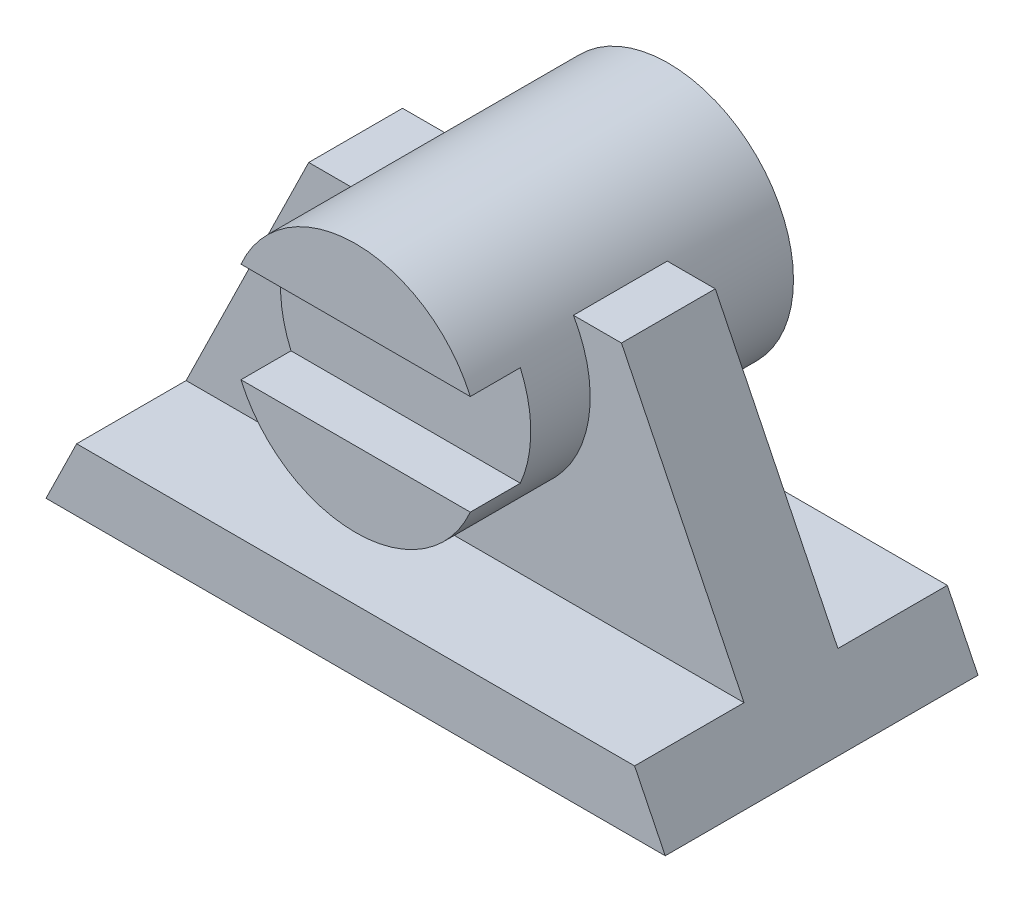
ISO-10303-21;
HEADER;
FILE_DESCRIPTION(('STEP AP214'),'2;1');
FILE_NAME('part.step','',(''),(''),'','','');
FILE_SCHEMA(('AUTOMOTIVE_DESIGN { 1 0 10303 214 1 1 1 1 }'));
ENDSEC;
DATA;
#1=APPLICATION_CONTEXT('core data for automotive mechanical design processes');
#2=APPLICATION_PROTOCOL_DEFINITION('international standard','automotive_design',2000,#1);
#3=PRODUCT_CONTEXT('',#1,'mechanical');
#4=PRODUCT('Part','Part','',(#3));
#5=PRODUCT_RELATED_PRODUCT_CATEGORY('part','',(#4));
#6=PRODUCT_DEFINITION_FORMATION('','',#4);
#7=PRODUCT_DEFINITION_CONTEXT('part definition',#1,'design');
#8=PRODUCT_DEFINITION('design','',#6,#7);
#9=PRODUCT_DEFINITION_SHAPE('','',#8);
#10=(LENGTH_UNIT() NAMED_UNIT(*) SI_UNIT(.MILLI.,.METRE.));
#11=(NAMED_UNIT(*) PLANE_ANGLE_UNIT() SI_UNIT($,.RADIAN.));
#12=(NAMED_UNIT(*) SI_UNIT($,.STERADIAN.) SOLID_ANGLE_UNIT());
#13=UNCERTAINTY_MEASURE_WITH_UNIT(LENGTH_MEASURE(1.E-05),#10,'distance_accuracy_value','');
#14=(GEOMETRIC_REPRESENTATION_CONTEXT(3) GLOBAL_UNCERTAINTY_ASSIGNED_CONTEXT((#13)) GLOBAL_UNIT_ASSIGNED_CONTEXT((#10,
#11,#12)) REPRESENTATION_CONTEXT('',''));
#15=CARTESIAN_POINT('',(0.,0.,0.));
#16=DIRECTION('',(0.,0.,1.));
#17=DIRECTION('',(1.,0.,0.));
#18=AXIS2_PLACEMENT_3D('',#15,#16,#17);
#19=CARTESIAN_POINT('',(0.,40.,25.));
#20=DIRECTION('',(0.,0.,1.));
#21=DIRECTION('',(1.,0.,0.));
#22=AXIS2_PLACEMENT_3D('',#19,#20,#21);
#23=PLANE('',#22);
#24=DIRECTION('',(-1.,0.,0.));
#25=VECTOR('',#24,1.);
#26=CARTESIAN_POINT('',(-23.6638655462185,48.,25.));
#27=LINE('',#26,#25);
#28=CARTESIAN_POINT('',(18.3303027798234,48.,25.));
#29=VERTEX_POINT('',#28);
#30=CARTESIAN_POINT('',(-18.3303027798234,48.,25.));
#31=VERTEX_POINT('',#30);
#32=EDGE_CURVE('E141',#29,#31,#27,.T.);
#33=ORIENTED_EDGE('',*,*,#32,.F.);
#34=CARTESIAN_POINT('',(0.,40.,25.));
#35=DIRECTION('',(0.,0.,1.));
#36=DIRECTION('',(1.,0.,0.));
#37=AXIS2_PLACEMENT_3D('',#34,#35,#36);
#38=CIRCLE('',#37,20.);
#39=EDGE_CURVE('E153',#29,#31,#38,.T.);
#40=ORIENTED_EDGE('',*,*,#39,.T.);
#41=EDGE_LOOP('',(#33,#40));
#42=FACE_BOUND('',#41,.T.);
#43=ADVANCED_FACE('F39',(#42),#23,.T.);
#44=CARTESIAN_POINT('',(0.,50.,0.));
#45=DIRECTION('',(0.,1.,0.));
#46=DIRECTION('',(0.,0.,1.));
#47=AXIS2_PLACEMENT_3D('',#44,#45,#46);
#48=PLANE('',#47);
#49=DIRECTION('',(-1.,0.,0.));
#50=VECTOR('',#49,1.);
#51=CARTESIAN_POINT('',(-49.5,50.,-7.50000000000001));
#52=LINE('',#51,#50);
#53=CARTESIAN_POINT('',(25.,50.,-7.50000000000001));
#54=VERTEX_POINT('',#53);
#55=CARTESIAN_POINT('',(17.3205080756888,50.,-7.50000000000001));
#56=VERTEX_POINT('',#55);
#57=EDGE_CURVE('E220',#54,#56,#52,.T.);
#58=ORIENTED_EDGE('',*,*,#57,.T.);
#59=DIRECTION('',(0.,0.,-1.));
#60=VECTOR('',#59,1.);
#61=CARTESIAN_POINT('',(17.3205080756888,50.,25.));
#62=LINE('',#61,#60);
#63=CARTESIAN_POINT('',(17.3205080756888,50.,7.49999999999999));
#64=VERTEX_POINT('',#63);
#65=EDGE_CURVE('E62',#56,#64,#62,.F.);
#66=ORIENTED_EDGE('',*,*,#65,.T.);
#67=DIRECTION('',(1.,0.,0.));
#68=VECTOR('',#67,1.);
#69=CARTESIAN_POINT('',(-49.5,50.,7.49999999999999));
#70=LINE('',#69,#68);
#71=CARTESIAN_POINT('',(25.,50.,7.49999999999999));
#72=VERTEX_POINT('',#71);
#73=EDGE_CURVE('E217',#64,#72,#70,.T.);
#74=ORIENTED_EDGE('',*,*,#73,.T.);
#75=DIRECTION('',(0.,0.,1.));
#76=VECTOR('',#75,1.);
#77=CARTESIAN_POINT('',(25.,50.,-40.));
#78=LINE('',#77,#76);
#79=EDGE_CURVE('E177',#54,#72,#78,.T.);
#80=ORIENTED_EDGE('',*,*,#79,.F.);
#81=EDGE_LOOP('',(#58,#66,#74,#80));
#82=FACE_BOUND('',#81,.T.);
#83=ADVANCED_FACE('F274',(#82),#48,.T.);
#84=CARTESIAN_POINT('',(-25.,50.,7.49999999999999));
#85=VERTEX_POINT('',#84);
#86=CARTESIAN_POINT('',(-17.3205080756888,50.,7.49999999999999));
#87=VERTEX_POINT('',#86);
#88=EDGE_CURVE('E215',#85,#87,#70,.T.);
#89=ORIENTED_EDGE('',*,*,#88,.T.);
#90=DIRECTION('',(0.,0.,-1.));
#91=VECTOR('',#90,1.);
#92=CARTESIAN_POINT('',(-17.3205080756888,50.,25.));
#93=LINE('',#92,#91);
#94=CARTESIAN_POINT('',(-17.3205080756888,50.,-7.50000000000001));
#95=VERTEX_POINT('',#94);
#96=EDGE_CURVE('E162',#87,#95,#93,.T.);
#97=ORIENTED_EDGE('',*,*,#96,.T.);
#98=CARTESIAN_POINT('',(-25.,50.,-7.50000000000001));
#99=VERTEX_POINT('',#98);
#100=EDGE_CURVE('E213',#95,#99,#52,.T.);
#101=ORIENTED_EDGE('',*,*,#100,.T.);
#102=DIRECTION('',(0.,0.,1.));
#103=VECTOR('',#102,1.);
#104=CARTESIAN_POINT('',(-25.,50.,-40.));
#105=LINE('',#104,#103);
#106=EDGE_CURVE('E179',#99,#85,#105,.T.);
#107=ORIENTED_EDGE('',*,*,#106,.T.);
#108=EDGE_LOOP('',(#89,#97,#101,#107));
#109=FACE_BOUND('',#108,.T.);
#110=ADVANCED_FACE('F279',(#109),#48,.T.);
#111=CARTESIAN_POINT('',(0.,10.,0.));
#112=DIRECTION('',(0.,1.,0.));
#113=DIRECTION('',(0.,0.,1.));
#114=AXIS2_PLACEMENT_3D('',#111,#112,#113);
#115=PLANE('',#114);
#116=DIRECTION('',(0.,0.,-1.));
#117=VECTOR('',#116,1.);
#118=CARTESIAN_POINT('',(-44.6,10.,0.));
#119=LINE('',#118,#117);
#120=CARTESIAN_POINT('',(-44.6,10.,-7.50000000000001));
#121=VERTEX_POINT('',#120);
#122=CARTESIAN_POINT('',(-44.6,10.,-25.));
#123=VERTEX_POINT('',#122);
#124=EDGE_CURVE('E199',#121,#123,#119,.T.);
#125=ORIENTED_EDGE('',*,*,#124,.F.);
#126=DIRECTION('',(-1.,0.,0.));
#127=VECTOR('',#126,1.);
#128=CARTESIAN_POINT('',(-49.5,10.,-7.50000000000001));
#129=LINE('',#128,#127);
#130=CARTESIAN_POINT('',(44.6,9.99999999999999,-7.50000000000001));
#131=VERTEX_POINT('',#130);
#132=EDGE_CURVE('E225',#131,#121,#129,.T.);
#133=ORIENTED_EDGE('',*,*,#132,.F.);
#134=DIRECTION('',(0.,0.,1.));
#135=VECTOR('',#134,1.);
#136=CARTESIAN_POINT('',(44.6,10.,0.));
#137=LINE('',#136,#135);
#138=CARTESIAN_POINT('',(44.6,10.,-25.));
#139=VERTEX_POINT('',#138);
#140=EDGE_CURVE('E182',#139,#131,#137,.T.);
#141=ORIENTED_EDGE('',*,*,#140,.F.);
#142=DIRECTION('',(-1.,0.,0.));
#143=VECTOR('',#142,1.);
#144=CARTESIAN_POINT('',(-49.5,10.,-25.));
#145=LINE('',#144,#143);
#146=EDGE_CURVE('E223',#139,#123,#145,.T.);
#147=ORIENTED_EDGE('',*,*,#146,.T.);
#148=EDGE_LOOP('',(#125,#133,#141,#147));
#149=FACE_BOUND('',#148,.T.);
#150=ADVANCED_FACE('F281',(#149),#115,.T.);
#151=CARTESIAN_POINT('',(-49.5,10.,-25.));
#152=DIRECTION('',(0.,0.,1.));
#153=DIRECTION('',(1.,0.,0.));
#154=AXIS2_PLACEMENT_3D('',#151,#152,#153);
#155=PLANE('',#154);
#156=DIRECTION('',(-1.,0.,0.));
#157=VECTOR('',#156,1.);
#158=CARTESIAN_POINT('',(-49.5,0.,-25.));
#159=LINE('',#158,#157);
#160=CARTESIAN_POINT('',(49.5,0.,-25.));
#161=VERTEX_POINT('',#160);
#162=CARTESIAN_POINT('',(-49.5,0.,-25.));
#163=VERTEX_POINT('',#162);
#164=EDGE_CURVE('E234',#161,#163,#159,.T.);
#165=ORIENTED_EDGE('',*,*,#164,.T.);
#166=DIRECTION('',(0.440015247772983,0.897990301577517,0.));
#167=VECTOR('',#166,1.);
#168=CARTESIAN_POINT('',(-45.5487057495363,8.0638658172728,-25.));
#169=LINE('',#168,#167);
#170=EDGE_CURVE('E198',#163,#123,#169,.T.);
#171=ORIENTED_EDGE('',*,*,#170,.T.);
#172=ORIENTED_EDGE('',*,*,#146,.F.);
#173=DIRECTION('',(0.440015247772983,-0.897990301577517,0.));
#174=VECTOR('',#173,1.);
#175=CARTESIAN_POINT('',(26.3809773405371,47.1816788968632,-25.));
#176=LINE('',#175,#174);
#177=EDGE_CURVE('E190',#139,#161,#176,.T.);
#178=ORIENTED_EDGE('',*,*,#177,.T.);
#179=EDGE_LOOP('',(#165,#171,#172,#178));
#180=FACE_BOUND('',#179,.T.);
#181=ADVANCED_FACE('F41',(#180),#155,.F.);
#182=CARTESIAN_POINT('',(-49.5,10.,25.));
#183=DIRECTION('',(0.,0.,-1.));
#184=DIRECTION('',(-1.,0.,0.));
#185=AXIS2_PLACEMENT_3D('',#182,#183,#184);
#186=PLANE('',#185);
#187=DIRECTION('',(1.,0.,0.));
#188=VECTOR('',#187,1.);
#189=CARTESIAN_POINT('',(-49.5,10.,25.));
#190=LINE('',#189,#188);
#191=CARTESIAN_POINT('',(-44.6,10.,25.));
#192=VERTEX_POINT('',#191);
#193=CARTESIAN_POINT('',(44.6,10.,25.));
#194=VERTEX_POINT('',#193);
#195=EDGE_CURVE('E226',#192,#194,#190,.T.);
#196=ORIENTED_EDGE('',*,*,#195,.F.);
#197=DIRECTION('',(-0.440015247772983,-0.897990301577517,0.));
#198=VECTOR('',#197,1.);
#199=CARTESIAN_POINT('',(-45.5487057495363,8.06386581727281,25.));
#200=LINE('',#199,#198);
#201=CARTESIAN_POINT('',(-49.5,0.,25.));
#202=VERTEX_POINT('',#201);
#203=EDGE_CURVE('E206',#192,#202,#200,.T.);
#204=ORIENTED_EDGE('',*,*,#203,.T.);
#205=DIRECTION('',(1.,0.,0.));
#206=VECTOR('',#205,1.);
#207=CARTESIAN_POINT('',(-49.5,0.,25.));
#208=LINE('',#207,#206);
#209=CARTESIAN_POINT('',(49.5,0.,25.));
#210=VERTEX_POINT('',#209);
#211=EDGE_CURVE('E230',#202,#210,#208,.T.);
#212=ORIENTED_EDGE('',*,*,#211,.T.);
#213=DIRECTION('',(-0.440015247772983,0.897990301577517,0.));
#214=VECTOR('',#213,1.);
#215=CARTESIAN_POINT('',(26.3809773405371,47.1816788968631,25.));
#216=LINE('',#215,#214);
#217=EDGE_CURVE('E193',#210,#194,#216,.T.);
#218=ORIENTED_EDGE('',*,*,#217,.T.);
#219=EDGE_LOOP('',(#196,#204,#212,#218));
#220=FACE_BOUND('',#219,.T.);
#221=ADVANCED_FACE('F305',(#220),#186,.F.);
#222=DIRECTION('',(0.,0.,-1.));
#223=VECTOR('',#222,1.);
#224=CARTESIAN_POINT('',(-44.6,10.,0.));
#225=LINE('',#224,#223);
#226=CARTESIAN_POINT('',(-44.6,10.,7.49999999999999));
#227=VERTEX_POINT('',#226);
#228=EDGE_CURVE('E207',#192,#227,#225,.T.);
#229=ORIENTED_EDGE('',*,*,#228,.F.);
#230=ORIENTED_EDGE('',*,*,#195,.T.);
#231=DIRECTION('',(0.,0.,1.));
#232=VECTOR('',#231,1.);
#233=CARTESIAN_POINT('',(44.6,10.,0.));
#234=LINE('',#233,#232);
#235=CARTESIAN_POINT('',(44.6,9.99999999999999,7.49999999999999));
#236=VERTEX_POINT('',#235);
#237=EDGE_CURVE('E194',#236,#194,#234,.T.);
#238=ORIENTED_EDGE('',*,*,#237,.F.);
#239=DIRECTION('',(1.,0.,0.));
#240=VECTOR('',#239,1.);
#241=CARTESIAN_POINT('',(-49.5,10.,7.49999999999999));
#242=LINE('',#241,#240);
#243=EDGE_CURVE('E212',#227,#236,#242,.T.);
#244=ORIENTED_EDGE('',*,*,#243,.F.);
#245=EDGE_LOOP('',(#229,#230,#238,#244));
#246=FACE_BOUND('',#245,.T.);
#247=ADVANCED_FACE('F299',(#246),#115,.T.);
#248=CARTESIAN_POINT('',(0.,0.,0.));
#249=DIRECTION('',(0.,1.,0.));
#250=DIRECTION('',(0.,0.,1.));
#251=AXIS2_PLACEMENT_3D('',#248,#249,#250);
#252=PLANE('',#251);
#253=DIRECTION('',(0.,0.,-1.));
#254=VECTOR('',#253,1.);
#255=CARTESIAN_POINT('',(49.5,0.,-25.));
#256=LINE('',#255,#254);
#257=EDGE_CURVE('E216',#210,#161,#256,.T.);
#258=ORIENTED_EDGE('',*,*,#257,.F.);
#259=ORIENTED_EDGE('',*,*,#211,.F.);
#260=DIRECTION('',(0.,0.,1.));
#261=VECTOR('',#260,1.);
#262=CARTESIAN_POINT('',(-49.5,0.,-25.));
#263=LINE('',#262,#261);
#264=EDGE_CURVE('E240',#163,#202,#263,.T.);
#265=ORIENTED_EDGE('',*,*,#264,.F.);
#266=ORIENTED_EDGE('',*,*,#164,.F.);
#267=EDGE_LOOP('',(#258,#259,#265,#266));
#268=FACE_BOUND('',#267,.T.);
#269=ADVANCED_FACE('F300',(#268),#252,.F.);
#270=CARTESIAN_POINT('',(-49.5,50.,7.49999999999999));
#271=DIRECTION('',(0.,0.,-1.));
#272=DIRECTION('',(-1.,0.,0.));
#273=AXIS2_PLACEMENT_3D('',#270,#271,#272);
#274=PLANE('',#273);
#275=CARTESIAN_POINT('',(0.,40.,7.49999999999999));
#276=DIRECTION('',(0.,0.,-1.));
#277=DIRECTION('',(-1.,0.,0.));
#278=AXIS2_PLACEMENT_3D('',#275,#276,#277);
#279=CIRCLE('',#278,20.);
#280=EDGE_CURVE('E176',#87,#64,#279,.F.);
#281=ORIENTED_EDGE('',*,*,#280,.F.);
#282=ORIENTED_EDGE('',*,*,#88,.F.);
#283=DIRECTION('',(-0.440015247772983,-0.897990301577517,0.));
#284=VECTOR('',#283,1.);
#285=CARTESIAN_POINT('',(-29.7435287476816,40.319329086364,7.49999999999999));
#286=LINE('',#285,#284);
#287=EDGE_CURVE('E204',#85,#227,#286,.T.);
#288=ORIENTED_EDGE('',*,*,#287,.T.);
#289=ORIENTED_EDGE('',*,*,#243,.T.);
#290=DIRECTION('',(-0.440015247772983,0.897990301577517,0.));
#291=VECTOR('',#290,1.);
#292=CARTESIAN_POINT('',(10.5758003386824,79.4371421659544,7.49999999999999));
#293=LINE('',#292,#291);
#294=EDGE_CURVE('E188',#236,#72,#293,.T.);
#295=ORIENTED_EDGE('',*,*,#294,.T.);
#296=ORIENTED_EDGE('',*,*,#73,.F.);
#297=EDGE_LOOP('',(#281,#282,#288,#289,#295,#296));
#298=FACE_BOUND('',#297,.T.);
#299=ADVANCED_FACE('F291',(#298),#274,.F.);
#300=CARTESIAN_POINT('',(-49.5,50.,-7.50000000000001));
#301=DIRECTION('',(0.,0.,1.));
#302=DIRECTION('',(1.,0.,0.));
#303=AXIS2_PLACEMENT_3D('',#300,#301,#302);
#304=PLANE('',#303);
#305=CARTESIAN_POINT('',(0.,40.,-7.50000000000001));
#306=DIRECTION('',(0.,0.,1.));
#307=DIRECTION('',(1.,0.,0.));
#308=AXIS2_PLACEMENT_3D('',#305,#306,#307);
#309=CIRCLE('',#308,20.);
#310=EDGE_CURVE('E244',#56,#95,#309,.F.);
#311=ORIENTED_EDGE('',*,*,#310,.F.);
#312=ORIENTED_EDGE('',*,*,#57,.F.);
#313=DIRECTION('',(0.440015247772983,-0.897990301577517,0.));
#314=VECTOR('',#313,1.);
#315=CARTESIAN_POINT('',(10.5758003386824,79.4371421659544,-7.50000000000001));
#316=LINE('',#315,#314);
#317=EDGE_CURVE('E235',#54,#131,#316,.T.);
#318=ORIENTED_EDGE('',*,*,#317,.T.);
#319=ORIENTED_EDGE('',*,*,#132,.T.);
#320=DIRECTION('',(0.440015247772983,0.897990301577517,0.));
#321=VECTOR('',#320,1.);
#322=CARTESIAN_POINT('',(-29.7435287476816,40.319329086364,-7.50000000000001));
#323=LINE('',#322,#321);
#324=EDGE_CURVE('E243',#121,#99,#323,.T.);
#325=ORIENTED_EDGE('',*,*,#324,.T.);
#326=ORIENTED_EDGE('',*,*,#100,.F.);
#327=EDGE_LOOP('',(#311,#312,#318,#319,#325,#326));
#328=FACE_BOUND('',#327,.T.);
#329=ADVANCED_FACE('F288',(#328),#304,.F.);
#330=CARTESIAN_POINT('',(25.,50.,-40.));
#331=DIRECTION('',(-0.897990301577517,-0.440015247772983,0.));
#332=DIRECTION('',(0.440015247772983,-0.897990301577517,0.));
#333=AXIS2_PLACEMENT_3D('',#330,#331,#332);
#334=PLANE('',#333);
#335=ORIENTED_EDGE('',*,*,#257,.T.);
#336=ORIENTED_EDGE('',*,*,#177,.F.);
#337=ORIENTED_EDGE('',*,*,#140,.T.);
#338=ORIENTED_EDGE('',*,*,#317,.F.);
#339=ORIENTED_EDGE('',*,*,#79,.T.);
#340=ORIENTED_EDGE('',*,*,#294,.F.);
#341=ORIENTED_EDGE('',*,*,#237,.T.);
#342=ORIENTED_EDGE('',*,*,#217,.F.);
#343=EDGE_LOOP('',(#335,#336,#337,#338,#339,#340,#341,#342));
#344=FACE_BOUND('',#343,.T.);
#345=ADVANCED_FACE('F289',(#344),#334,.F.);
#346=CARTESIAN_POINT('',(-25.,50.,-40.));
#347=DIRECTION('',(0.897990301577517,-0.440015247772983,0.));
#348=DIRECTION('',(0.440015247772983,0.897990301577517,0.));
#349=AXIS2_PLACEMENT_3D('',#346,#347,#348);
#350=PLANE('',#349);
#351=ORIENTED_EDGE('',*,*,#228,.T.);
#352=ORIENTED_EDGE('',*,*,#287,.F.);
#353=ORIENTED_EDGE('',*,*,#106,.F.);
#354=ORIENTED_EDGE('',*,*,#324,.F.);
#355=ORIENTED_EDGE('',*,*,#124,.T.);
#356=ORIENTED_EDGE('',*,*,#170,.F.);
#357=ORIENTED_EDGE('',*,*,#264,.T.);
#358=ORIENTED_EDGE('',*,*,#203,.F.);
#359=EDGE_LOOP('',(#351,#352,#353,#354,#355,#356,#357,#358));
#360=FACE_BOUND('',#359,.T.);
#361=ADVANCED_FACE('F268',(#360),#350,.F.);
#362=CARTESIAN_POINT('',(0.,40.,25.));
#363=DIRECTION('',(0.,0.,-1.));
#364=DIRECTION('',(-1.,0.,0.));
#365=AXIS2_PLACEMENT_3D('',#362,#363,#364);
#366=CYLINDRICAL_SURFACE('',#365,20.);
#367=CARTESIAN_POINT('',(-18.3303027798234,32.,25.));
#368=VERTEX_POINT('',#367);
#369=CARTESIAN_POINT('',(18.3303027798234,32.,25.));
#370=VERTEX_POINT('',#369);
#371=EDGE_CURVE('E161',#368,#370,#38,.T.);
#372=ORIENTED_EDGE('',*,*,#371,.F.);
#373=DIRECTION('',(0.,0.,-1.));
#374=VECTOR('',#373,1.);
#375=CARTESIAN_POINT('',(-18.3303027798234,32.,25.));
#376=LINE('',#375,#374);
#377=CARTESIAN_POINT('',(-18.3303027798234,32.,17.));
#378=VERTEX_POINT('',#377);
#379=EDGE_CURVE('E171',#368,#378,#376,.T.);
#380=ORIENTED_EDGE('',*,*,#379,.T.);
#381=CARTESIAN_POINT('',(0.,40.,17.));
#382=DIRECTION('',(0.,0.,1.));
#383=DIRECTION('',(1.,0.,0.));
#384=AXIS2_PLACEMENT_3D('',#381,#382,#383);
#385=CIRCLE('',#384,20.);
#386=CARTESIAN_POINT('',(-18.3303027798234,48.,17.));
#387=VERTEX_POINT('',#386);
#388=EDGE_CURVE('E11',#387,#378,#385,.T.);
#389=ORIENTED_EDGE('',*,*,#388,.F.);
#390=DIRECTION('',(0.,0.,-1.));
#391=VECTOR('',#390,1.);
#392=CARTESIAN_POINT('',(-18.3303027798234,48.,25.));
#393=LINE('',#392,#391);
#394=EDGE_CURVE('E152',#387,#31,#393,.F.);
#395=ORIENTED_EDGE('',*,*,#394,.T.);
#396=ORIENTED_EDGE('',*,*,#39,.F.);
#397=DIRECTION('',(0.,0.,-1.));
#398=VECTOR('',#397,1.);
#399=CARTESIAN_POINT('',(18.3303027798234,48.,25.));
#400=LINE('',#399,#398);
#401=CARTESIAN_POINT('',(18.3303027798234,48.,17.));
#402=VERTEX_POINT('',#401);
#403=EDGE_CURVE('E138',#29,#402,#400,.T.);
#404=ORIENTED_EDGE('',*,*,#403,.T.);
#405=CARTESIAN_POINT('',(18.3303027798234,32.,17.));
#406=VERTEX_POINT('',#405);
#407=EDGE_CURVE('E43',#406,#402,#385,.T.);
#408=ORIENTED_EDGE('',*,*,#407,.F.);
#409=DIRECTION('',(0.,0.,-1.));
#410=VECTOR('',#409,1.);
#411=CARTESIAN_POINT('',(18.3303027798234,32.,25.));
#412=LINE('',#411,#410);
#413=EDGE_CURVE('E148',#406,#370,#412,.F.);
#414=ORIENTED_EDGE('',*,*,#413,.T.);
#415=EDGE_LOOP('',(#372,#380,#389,#395,#396,#404,#408,#414));
#416=FACE_BOUND('',#415,.T.);
#417=CARTESIAN_POINT('',(0.,40.,-25.));
#418=DIRECTION('',(0.,0.,1.));
#419=DIRECTION('',(1.,0.,0.));
#420=AXIS2_PLACEMENT_3D('',#417,#418,#419);
#421=CIRCLE('',#420,20.);
#422=CARTESIAN_POINT('',(20.,40.,-25.));
#423=VERTEX_POINT('',#422);
#424=EDGE_CURVE('E166',#423,#423,#421,.T.);
#425=ORIENTED_EDGE('',*,*,#424,.T.);
#426=EDGE_LOOP('',(#425));
#427=FACE_BOUND('',#426,.T.);
#428=ORIENTED_EDGE('',*,*,#96,.F.);
#429=ORIENTED_EDGE('',*,*,#280,.T.);
#430=ORIENTED_EDGE('',*,*,#65,.F.);
#431=ORIENTED_EDGE('',*,*,#310,.T.);
#432=EDGE_LOOP('',(#428,#429,#430,#431));
#433=FACE_BOUND('',#432,.T.);
#434=ADVANCED_FACE('F156',(#416,#427,#433),#366,.T.);
#435=DIRECTION('',(1.,0.,0.));
#436=VECTOR('',#435,1.);
#437=CARTESIAN_POINT('',(-23.6638655462185,32.,25.));
#438=LINE('',#437,#436);
#439=EDGE_CURVE('E157',#368,#370,#438,.T.);
#440=ORIENTED_EDGE('',*,*,#439,.F.);
#441=ORIENTED_EDGE('',*,*,#371,.T.);
#442=EDGE_LOOP('',(#440,#441));
#443=FACE_BOUND('',#442,.T.);
#444=ADVANCED_FACE('F259',(#443),#23,.T.);
#445=CARTESIAN_POINT('',(0.,40.,-25.));
#446=DIRECTION('',(0.,0.,1.));
#447=DIRECTION('',(1.,0.,0.));
#448=AXIS2_PLACEMENT_3D('',#445,#446,#447);
#449=PLANE('',#448);
#450=ORIENTED_EDGE('',*,*,#424,.F.);
#451=EDGE_LOOP('',(#450));
#452=FACE_BOUND('',#451,.T.);
#453=ADVANCED_FACE('F258',(#452),#449,.F.);
#454=CARTESIAN_POINT('',(0.,0.,17.));
#455=DIRECTION('',(0.,0.,1.));
#456=DIRECTION('',(1.,0.,0.));
#457=AXIS2_PLACEMENT_3D('',#454,#455,#456);
#458=PLANE('',#457);
#459=ORIENTED_EDGE('',*,*,#388,.T.);
#460=DIRECTION('',(1.,0.,0.));
#461=VECTOR('',#460,1.);
#462=CARTESIAN_POINT('',(-23.6638655462185,32.,17.));
#463=LINE('',#462,#461);
#464=EDGE_CURVE('E52',#378,#406,#463,.T.);
#465=ORIENTED_EDGE('',*,*,#464,.T.);
#466=ORIENTED_EDGE('',*,*,#407,.T.);
#467=DIRECTION('',(-1.,0.,0.));
#468=VECTOR('',#467,1.);
#469=CARTESIAN_POINT('',(-23.6638655462185,48.,17.));
#470=LINE('',#469,#468);
#471=EDGE_CURVE('E147',#402,#387,#470,.T.);
#472=ORIENTED_EDGE('',*,*,#471,.T.);
#473=EDGE_LOOP('',(#459,#465,#466,#472));
#474=FACE_BOUND('',#473,.T.);
#475=ADVANCED_FACE('F270',(#474),#458,.T.);
#476=CARTESIAN_POINT('',(-23.6638655462185,32.,17.));
#477=DIRECTION('',(0.,-1.,0.));
#478=DIRECTION('',(0.,0.,-1.));
#479=AXIS2_PLACEMENT_3D('',#476,#477,#478);
#480=PLANE('',#479);
#481=ORIENTED_EDGE('',*,*,#439,.T.);
#482=ORIENTED_EDGE('',*,*,#413,.F.);
#483=ORIENTED_EDGE('',*,*,#464,.F.);
#484=ORIENTED_EDGE('',*,*,#379,.F.);
#485=EDGE_LOOP('',(#481,#482,#483,#484));
#486=FACE_BOUND('',#485,.T.);
#487=ADVANCED_FACE('F257',(#486),#480,.F.);
#488=CARTESIAN_POINT('',(-23.6638655462185,48.,17.));
#489=DIRECTION('',(0.,1.,0.));
#490=DIRECTION('',(0.,0.,1.));
#491=AXIS2_PLACEMENT_3D('',#488,#489,#490);
#492=PLANE('',#491);
#493=ORIENTED_EDGE('',*,*,#32,.T.);
#494=ORIENTED_EDGE('',*,*,#394,.F.);
#495=ORIENTED_EDGE('',*,*,#471,.F.);
#496=ORIENTED_EDGE('',*,*,#403,.F.);
#497=EDGE_LOOP('',(#493,#494,#495,#496));
#498=FACE_BOUND('',#497,.T.);
#499=ADVANCED_FACE('F145',(#498),#492,.F.);
#500=CLOSED_SHELL('',(#43,#83,#110,#150,#181,#221,#247,#269,#299,#329,#345,#361,#434,#444,#453,
#475,#487,#499));
#501=MANIFOLD_SOLID_BREP('B2',#500);
#502=ADVANCED_BREP_SHAPE_REPRESENTATION('',(#18,#501),#14);
#503=SHAPE_DEFINITION_REPRESENTATION(#9,#502);
ENDSEC;
END-ISO-10303-21;
